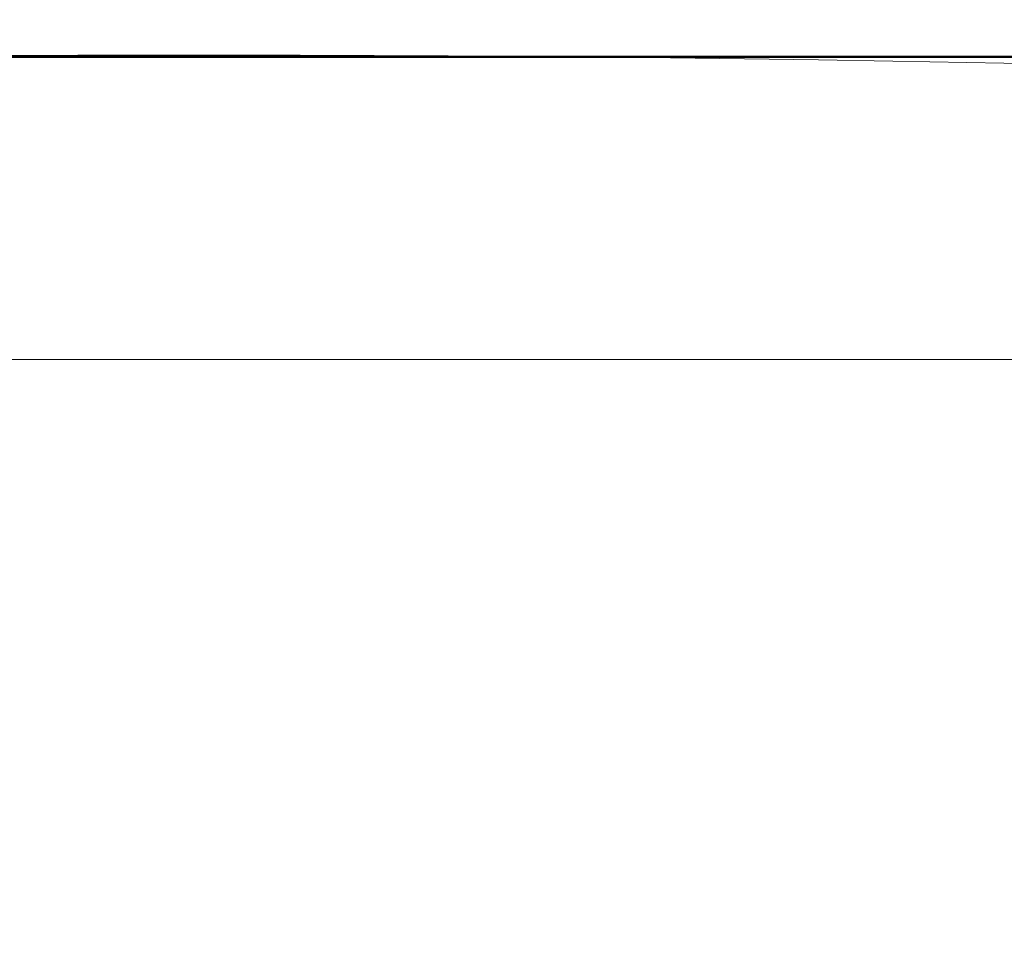
# Model space of a CAD drawing. Units: inches. Extents: x -466983 to 1020, y 324 to 318697.
# Tile 73 of 97: x 643.839 to 650.415, y 947.975 to 954.185. Entities that reach past the tile are written whole.
import ezdxf

# ---------------------------------------------------------------- set-up
doc = ezdxf.new("R2010")
doc.units = ezdxf.units.IN
doc.header["$MEASUREMENT"] = 0
for name, color, linetype, lineweight in [('A-FLOR-PATT', 252, 'Continuous', 13), ('A-FURN', 8, 'Continuous', 18), ('A-WALL', 7, 'Continuous', 50)]:
    doc.layers.add(name, color=color, linetype=linetype, lineweight=lineweight)

# ---------------------------------------------------------------- blocks, each defined once
blk = doc.blocks.new('L Shaped Sofa')
at = {"ltscale": 2}
for p, q in [((2430.914, 726.917), (2396.145, 726.917)), ((2475.263, 723.229), (2377.232, 723.229))]:
    blk.add_line(p, q, dxfattribs=at)
blk.add_arc((2416.36, 1205.029), 481.82, 262.88673, 276.63201, dxfattribs=at)

msp = doc.modelspace()

# ---------------------------------------------------------------- hatches: boundary and pattern name
at = {"layer": 'A-FLOR-PATT', "transparency": 33554572}
h = msp.add_hatch(dxfattribs=at)
h.set_pattern_fill('ANSI37', color=256, scale=30)
h.set_pattern_definition([(45, (-1212.4137, -290.035), (-2.6516504, 2.6516504), []), (135, (-1212.4137, -290.035), (-2.6516504, -2.6516504), [])])
h.paths.add_polyline_path([(901.8057, 1075.9377), (900.6144, 1075.9377), (900.6144, 1065.3856), (899.391, 1065.3856), (898.0911, 1065.3856), (892.8356, 1058.7098, -0.258377), (892.1875, 1058.3509), (879.9848, 1058.3509, -0.20177), (879.4382, 1058.5808), (874.0812, 1065.3856), (872.7813, 1065.3856), (871.5579, 1065.3856), (871.5579, 1075.9377), (813.8057, 1075.9377), (813.8057, 1044.7922), (832.3947, 1044.7922, -0.394795), (848.6602, 1028.5356), (848.6602, 1009.9377), (901.8057, 1009.9377), (901.8057, 1015.9377), (901.3057, 1015.9377), (871.3057, 1015.9377), (871.3057, 1017.2502), (871.3344, 1017.2502, -0.401453), (901.3057, 1045.9377), (901.8057, 1045.9377)])
edge = h.paths.add_edge_path(flags=16)
edge.add_line((847.7731, 1068.9486), (847.7731, 1073.7088))
edge.add_arc((849.2269, 1073.7088), 1.4538, 90, 180, ccw=False)
edge.add_line((849.2269, 1075.1627), (864.4921, 1075.1627))
edge.add_arc((864.4921, 1073.7088), 1.4538, 0, 90, ccw=False)
edge.add_line((865.9459, 1073.7088), (865.9459, 1069.0035))
edge.add_arc((832.6447, 1068.9761), 33.3012, -20.61234, 0.04725, ccw=False)
edge.add_ellipse((856.8595, 1058.48), major_axis=(0, 10.2131), ratio=0.6859192, start_angle=100.00884, end_angle=259.99116, ccw=False)
edge.add_arc((881.0742, 1068.9761), 33.3012, 180.04725, 200.61234, ccw=False)
h.paths.add_polyline_path([(853.1456, 1066.4815), (853.1456, 1066.4534), (853.1463, 1066.4534, 0.433107), (852.9166, 1066.6849), (852.9166, 1066.4534), (853.1456, 1066.4534), (853.1456, 1066.4815), (853.088, 1066.6122, 0.697939), (852.6995, 1066.4534), (852.7003, 1066.4534), (852.7003, 1066.4815), (852.9166, 1067.0012), (852.9166, 1066.6849, -0.396254)], flags=0)
h.paths.add_polyline_path([(861.0187, 1066.4815), (861.0187, 1066.4534), (861.0194, 1066.4534, 0.416404), (860.8024, 1066.6849), (860.8024, 1066.4534), (861.0187, 1066.4534), (861.0187, 1066.4815), (860.9672, 1066.6053, 0.713344), (860.5726, 1066.4534), (860.5734, 1066.4534), (860.5734, 1066.4815), (860.8024, 1067.0012), (860.8024, 1066.6849, -0.379973)], flags=0)
edge = h.paths.add_edge_path(flags=0)
edge.add_spline(control_points=[(861.1298, 1065.7855), (861.4661, 1065.2478), (861.6134, 1065.0161), (861.9833, 1064.3736), (862.1924, 1063.9443), (862.5614, 1063.0391), (862.7212, 1062.5633), (862.9865, 1061.5781), (863.092, 1061.0689), (863.2452, 1060.031), (863.293, 1059.5025), (863.3295, 1058.4409), (863.3181, 1057.9078), (863.2366, 1056.8518), (863.1664, 1056.3289), (862.9695, 1055.308), (862.8427, 1054.8099), (862.5365, 1053.8522), (862.3571, 1053.3927), (861.9514, 1052.5249), (861.7251, 1052.1166), (861.233, 1051.3622), (860.9672, 1051.0162), (860.4048, 1050.3949), (860.1082, 1050.1197), (859.4937, 1049.6461), (859.1758, 1049.4476), (858.5276, 1049.1299), (858.1973, 1049.0107), (857.5315, 1048.8518), (857.1959, 1048.8121), (856.5249, 1048.812), (856.1894, 1048.8515), (855.5236, 1049.0101), (855.1933, 1049.1291), (854.545, 1049.4465), (854.2271, 1049.6449), (853.6124, 1050.1183), (853.3158, 1050.3933), (852.7533, 1051.0143), (852.4874, 1051.3602), (851.9952, 1052.1144), (851.7688, 1052.5225), (851.3629, 1053.3902), (851.1834, 1053.8496), (850.877, 1054.8071), (850.7501, 1055.3051), (850.553, 1056.326), (850.4827, 1056.8488), (850.401, 1057.9048), (850.3895, 1058.4379), (850.4257, 1059.4995), (850.4734, 1060.0281), (850.6265, 1061.066), (850.7318, 1061.5753), (850.9969, 1062.5605), (851.1567, 1063.0365), (851.5254, 1063.9418), (851.7345, 1064.3712), (852.1056, 1065.0164), (852.2544, 1065.2503), (852.6082, 1065.7335)], knot_values=[3.915332, 3.915332, 3.915332, 3.915332, 4.013468, 4.013468, 4.175532, 4.175532, 4.337596, 4.337596, 4.49966, 4.49966, 4.661724, 4.661724, 4.823788, 4.823788, 4.985852, 4.985852, 5.147916, 5.147916, 5.30998, 5.30998, 5.472044, 5.472044, 5.634109, 5.634109, 5.796173, 5.796173, 5.958237, 5.958237, 6.120301, 6.120301, 6.282365, 6.282365, 6.444429, 6.444429, 6.606493, 6.606493, 6.768557, 6.768557, 6.930621, 6.930621, 7.092685, 7.092685, 7.254749, 7.254749, 7.416813, 7.416813, 7.578878, 7.578878, 7.740942, 7.740942, 7.903006, 7.903006, 8.06507, 8.06507, 8.227134, 8.227134, 8.389198, 8.389198, 8.551262, 8.551262, 8.65037, 8.65037, 8.65037, 8.65037], degree=3, periodic=0)
edge.add_line((852.6421, 1065.7855), (861.1298, 1065.7855))
edge = h.paths.add_edge_path(flags=0)
edge.add_ellipse((856.8496, 1057.7432), major_axis=(0, 7.7921), ratio=0.687861, start_angle=0, end_angle=360)
h.paths.add_polyline_path([(848.8634, 1069.3891), (848.8634, 1073.9605, -0.414214), (849.9538, 1075.0508), (863.7652, 1075.0508, -0.414214), (864.8555, 1073.9605), (864.8555, 1069.3891, -0.388936), (864.5237, 1069.027, -0.043561), (849.1953, 1069.027, -0.388936)], flags=0)
h.paths.add_polyline_path([(853.1006, 1068.1122, -1), (852.6775, 1068.1122, -1)], flags=0)
edge = h.paths.add_edge_path(flags=0)
edge.add_ellipse((856.8595, 1057.3378), major_axis=(0, 2.207), ratio=0.657164, start_angle=0, end_angle=360)
h.paths.add_polyline_path([(861.0415, 1068.1122, -1), (860.6184, 1068.1122, -1)], flags=0)
edge = h.paths.add_edge_path()
edge.add_line((573.9537, 1057.3412), (573.9537, 1075.9377))
edge.add_line((573.9537, 1075.9377), (558.7308, 1075.9377))
edge.add_line((558.7308, 1075.9377), (558.7308, 1065.3856))
edge.add_line((558.7308, 1065.3856), (557.5074, 1065.3856))
edge.add_line((557.5074, 1065.3856), (556.2075, 1065.3856))
edge.add_line((556.2075, 1065.3856), (550.952, 1058.7098))
edge.add_arc((550.3039, 1059.1155), 0.7646, 270, 327.94832, ccw=False)
edge.add_line((550.3039, 1058.3509), (538.1012, 1058.3509))
edge.add_arc((538.1012, 1059.1155), 0.7646, 224.3704, 270, ccw=False)
edge.add_line((537.5546, 1058.5808), (532.1976, 1065.3856))
edge.add_line((532.1976, 1065.3856), (530.8977, 1065.3856))
edge.add_line((530.8977, 1065.3856), (529.6743, 1065.3856))
edge.add_line((529.6743, 1065.3856), (529.6743, 1075.9377))
edge.add_line((529.6743, 1075.9377), (520.8057, 1075.9377))
edge.add_line((520.8057, 1075.9377), (520.8057, 1045.9377))
edge.add_line((520.8057, 1045.9377), (521.3057, 1045.9377))
edge.add_arc((521.3057, 1015.9377), 30, 2.50749, 90, ccw=False)
edge.add_line((551.277, 1017.2502), (551.3057, 1017.2502))
edge.add_line((551.3057, 1017.2502), (551.3057, 1015.9377))
edge.add_line((551.3057, 1015.9377), (520.8057, 1015.9377))
edge.add_line((520.8057, 1015.9377), (520.8057, 1009.9377))
edge.add_line((520.8057, 1009.9377), (559.1913, 1010.4022))
edge.add_arc((559.1913, 1011.856), 1.4538, 180, 270, ccw=False)
edge.add_line((557.7375, 1011.856), (557.7375, 1016.5613))
edge.add_arc((591.0386, 1016.5888), 33.3012, 159.38766, 180.04725, ccw=False)
edge.add_ellipse((566.8239, 1027.0848), major_axis=(0, 10.2131), ratio=0.6859192, start_angle=280.00884, end_angle=439.99116, ccw=False)
edge.add_arc((542.6091, 1016.5888), 33.3012, 0.04725, 20.61234, ccw=False)
edge.add_line((575.9103, 1016.6162), (575.9103, 1011.856))
edge.add_arc((574.4565, 1011.856), 1.4538, -90, 0, ccw=False)
edge.add_line((574.4565, 1010.4022), (608.8057, 1009.9377))
edge.add_line((608.8057, 1009.9377), (608.8057, 1041.0857))
edge.add_line((608.8057, 1041.0857), (590.2179, 1041.0857))
edge.add_arc((590.775, 1057.9074), 16.8309, 181.92775, 268.10321, ccw=False)
edge = h.paths.add_edge_path()
edge.add_ellipse((494.2443, 583.6204), major_axis=(0, 10.2131), ratio=0.6859192, start_angle=280.00884, end_angle=439.99116, ccw=False)
edge.add_arc((470.0296, 573.1243), 33.3012, 0.04725, 20.61234, ccw=False)
edge.add_line((503.3307, 573.1518), (503.3307, 568.3916))
edge.add_arc((501.8769, 568.3916), 1.4538, -90, 0, ccw=False)
edge.add_line((501.8769, 566.9377), (539.8057, 566.9377))
edge.add_line((539.8057, 566.9377), (539.8057, 572.9377))
edge.add_line((539.8057, 572.9377), (539.3057, 572.9377))
edge.add_line((539.3057, 572.9377), (509.3057, 572.9377))
edge.add_line((509.3057, 572.9377), (509.3057, 574.2502))
edge.add_line((509.3057, 574.2502), (509.3344, 574.2502))
edge.add_arc((539.3057, 572.9377), 30, 90, 177.49251, ccw=False)
edge.add_line((539.3057, 602.9377), (539.8057, 602.9377))
edge.add_line((539.8057, 602.9377), (539.8057, 626.9377))
edge.add_line((539.8057, 626.9377), (531.7718, 626.9377))
edge.add_line((531.7718, 626.9377), (531.7718, 616.3856))
edge.add_line((531.7718, 616.3856), (530.5484, 616.3856))
edge.add_line((530.5484, 616.3856), (529.2485, 616.3856))
edge.add_line((529.2485, 616.3856), (523.7105, 609.3509))
edge.add_line((523.7105, 609.3509), (510.7766, 609.3509))
edge.add_line((510.7766, 609.3509), (505.2386, 616.3856))
edge.add_line((505.2386, 616.3856), (503.9387, 616.3856))
edge.add_line((503.9387, 616.3856), (502.7153, 616.3856))
edge.add_line((502.7153, 616.3856), (502.7153, 626.9377))
edge.add_line((502.7153, 626.9377), (481.6983, 626.9377))
edge.add_line((481.6983, 626.9377), (481.6983, 610.995))
edge.add_arc((467.2703, 611.4728), 14.4359, 271.92775, 358.10321, ccw=False)
edge.add_line((467.7559, 597.0451), (451.8057, 597.0451))
edge.add_line((451.8057, 597.0451), (451.8057, 584.4035))
edge.add_line((451.8057, 584.4035), (451.8057, 566.9377))
edge.add_line((451.8057, 566.9377), (486.6117, 566.9377))
edge.add_arc((486.6117, 568.3916), 1.4538, 180, 270, ccw=False)
edge.add_line((485.1579, 568.3916), (485.1579, 573.0969))
edge.add_arc((518.4591, 573.1243), 33.3012, 159.38766, 180.04725, ccw=False)
h.paths.add_polyline_path([(836.2609, 1020.7328), (879.8898, 1020.7328), (879.8898, 1039.3902), (836.2609, 1039.3902)], flags=25)
h.paths.add_polyline_path([(549.9851, 1036.7492), (593.614, 1036.7492), (593.614, 1055.4065), (549.9851, 1055.4065)], flags=24)
h.paths.add_polyline_path([(475.123, 595.5959), (518.752, 595.5959), (518.752, 614.2532), (475.123, 614.2532)], flags=24)
h = msp.add_hatch(dxfattribs=at)
h.set_pattern_fill('ANSI37', color=256, scale=20)
h.set_pattern_definition([(45, (-1212.4137, -290.035), (-1.767767, 1.767767), []), (135, (-1212.4137, -290.035), (-1.767767, -1.767767), [])])
h.paths.add_polyline_path([(809.8057, 870.9377), (809.8057, 888.1519), (806.9985, 888.1519), (802.6624, 888.1519), (789.3832, 888.1519), (786.2846, 888.1519, -0.414214), (785.4991, 888.9374), (785.4991, 900.1959), (785.4991, 908.4696, -0.414214), (786.8082, 909.7787, -0.414214), (785.4991, 911.0878), (785.4991, 929.1015, -0.414214), (786.8082, 930.4106, -0.414214), (785.4991, 931.7197), (785.4991, 931.9039, -0.414214), (784.19, 930.5948), (766.7223, 930.5948, -0.412359), (765.4132, 931.8956, -0.413741), (764.1145, 930.5782), (744.5781, 930.422, -0.416556), (743.7864, 931.2075), (743.7864, 933.5153), (742.2154, 933.5153), (742.2154, 952.024, -0.001344), (743.7864, 952.1998), (743.7864, 953.9377), (678.5915, 953.9377), (678.5915, 951.1305), (678.5915, 946.7945), (678.5915, 933.5153), (678.5915, 930.4166, -0.414214), (677.806, 929.6312), (666.5475, 929.6312), (658.2738, 929.6312, -0.414214), (656.9647, 930.9403, -0.414214), (655.6556, 929.6312), (637.6419, 929.6312, -0.414214), (636.3328, 930.9403, -0.414214), (635.0237, 929.6312), (634.8395, 929.6312, -0.414214), (636.1486, 928.322), (636.1486, 910.8544, -0.412359), (634.8478, 909.5452, -0.413741), (636.1653, 908.2466), (636.3214, 888.7102, -0.416556), (635.5359, 887.9184), (633.2281, 887.9184), (633.2281, 886.3475), (614.7194, 886.3475, -0.001344), (614.5436, 887.9184), (612.8057, 887.9184), (612.8057, 834.9377), (612.8057, 752.9377), (612.8057, 748.9377), (612.8057, 697.9377), (654.8057, 697.9377), (654.8057, 701.9377), (715.8057, 701.9377), (715.8057, 737.4353), (774.2918, 737.4353), (774.2918, 795.9377), (809.8057, 795.9377)])
h.paths.add_polyline_path([(679.2761, 849.5757, 0.102523), (682.1475, 849.2608, -0.080461), (694.5428, 849.7725, -0.283899), (694.4822, 849.0082, 0.136605), (694.4068, 848.8103, -0.030441), (694.5428, 846.8929), (694.5428, 842.6198), (694.5428, 838.3466, -0.028219), (694.4246, 836.5684), (694.425, 836.5684, 0.196187), (694.4456, 836.2708, -0.302897), (694.5428, 835.467, -0.080461), (682.1475, 835.9787, 0.102523), (679.2761, 835.6638, -0.58611), (678.6457, 836.0169), (678.6457, 849.2227, -0.58611)], flags=16)
h.paths.add_polyline_path([(679.5173, 848.6515, 0.699597), (679.476, 848.6342, 1.20716), (679.1935, 848.7422, 0.010621)], flags=0)
h.paths.add_polyline_path([(679.4923, 836.5608, -0.013798), (679.9178, 836.6594, -0.071703), (682.8533, 837.1434, -0.165743), (682.1665, 839.1006), (682.1665, 842.6094), (682.1665, 846.0603, -0.240616), (683.4733, 848.6767, -0.068263), (693.9295, 849.0082), (693.7875, 848.7083), (693.7875, 849.0228, 0.067332), (683.4733, 848.6767, 0.240616), (682.1665, 846.0603), (682.1665, 842.6094), (682.1665, 839.1006, 0.23459), (683.461, 836.5513, 0.068093), (693.7875, 836.1955), (693.7875, 836.5104), (693.9296, 836.2102, -0.077215), (682.2421, 836.7815, 0.086627), (679.5283, 836.5701, -0.628402), (679.5029, 836.5735), (679.5029, 836.6071, 0.910458)], flags=0)
h.paths.add_polyline_path([(679.476, 848.6364), (679.2069, 848.647), (679.2069, 836.5718, 0.913566), (679.3645, 836.5861), (679.476, 836.5824)], flags=0)
h.paths.add_polyline_path([(679.2761, 829.8604, 0.102523), (682.1475, 829.5455, -0.080461), (694.5428, 830.0572, -0.283899), (694.4822, 829.2929, 0.136605), (694.4068, 829.095, -0.030441), (694.5428, 827.1776), (694.5428, 822.9045), (694.5428, 818.6314, -0.028219), (694.4246, 816.8531), (694.425, 816.8532, 0.196187), (694.4456, 816.5555, -0.302897), (694.5428, 815.7517, -0.080461), (682.1475, 816.2635, 0.102523), (679.2761, 815.9485, -0.58611), (678.6457, 816.3016), (678.6457, 829.5074, -0.58611)], flags=16)
h.paths.add_polyline_path([(679.5173, 828.9362, 0.699597), (679.476, 828.9189, 1.20716), (679.1935, 829.0269, 0.010621)], flags=0)
h.paths.add_polyline_path([(679.4923, 816.8456, -0.013798), (679.9178, 816.9441, -0.071703), (682.8533, 817.4281, -0.165743), (682.1665, 819.3853), (682.1665, 822.8941), (682.1665, 826.345, -0.240616), (683.4733, 828.9614, -0.068263), (693.9295, 829.2929), (693.7875, 828.9931), (693.7875, 829.3076, 0.067332), (683.4733, 828.9614, 0.240616), (682.1665, 826.345), (682.1665, 822.8941), (682.1665, 819.3853, 0.23459), (683.461, 816.836, 0.068093), (693.7875, 816.4802), (693.7875, 816.7952), (693.9296, 816.4949, -0.077215), (682.2421, 817.0662, 0.086627), (679.5283, 816.8549, -0.628402), (679.5029, 816.8582), (679.5029, 816.8918, 0.910458)], flags=0)
h.paths.add_polyline_path([(679.476, 828.9211), (679.2069, 828.9317), (679.2069, 816.8565, 0.913566), (679.3645, 816.8708), (679.476, 816.8671)], flags=0)
h.paths.add_polyline_path([(679.2761, 810.1451, 0.102523), (682.1475, 809.8302, -0.080461), (694.5428, 810.342, -0.3023), (694.4466, 809.5394, 0.10023), (694.4058, 809.3878, -0.03057), (694.5428, 807.4623), (694.5428, 803.1892), (694.5428, 798.9161, -0.03057), (694.4058, 796.9906, 0.10023), (694.4466, 796.839, -0.3023), (694.5428, 796.0365, -0.080461), (682.1475, 796.5482, 0.102523), (679.2761, 796.2333, -0.58611), (678.6457, 796.5863), (678.6457, 809.7921, -0.58611)], flags=16)
h.paths.add_polyline_path([(679.5173, 809.2417, 0.699597), (679.476, 809.2244, 1.20716), (679.1935, 809.3324, 0.010621)], flags=0)
h.paths.add_polyline_path([(679.4923, 797.151, -0.013798), (679.9178, 797.2496, -0.071703), (682.8533, 797.7336, -0.165743), (682.1665, 799.6908), (682.1665, 803.1996), (682.1665, 806.6505, -0.239349), (683.461, 809.2577, -0.072465), (694.4468, 809.5405, 0.197932), (694.425, 809.2405), (693.7875, 809.2985), (693.7875, 809.6135, 0.068093), (683.461, 809.2577, 0.239349), (682.1665, 806.6505), (682.1665, 803.1996), (682.1665, 799.6908, 0.235854), (683.4733, 797.1323, 0.067332), (693.7875, 796.7861), (693.7875, 797.1006), (694.425, 797.1586, 0.197932), (694.4468, 796.8586, -0.080419), (682.1557, 797.3795, 0.083867), (679.5283, 797.1603, -0.628402), (679.5029, 797.1637), (679.5029, 797.1973, 0.910458)], flags=0)
h.paths.add_polyline_path([(679.2069, 809.2372), (679.2069, 797.162, 0.913566), (679.3645, 797.1763), (679.476, 797.1726), (679.476, 809.2266)], flags=0)
h.paths.add_polyline_path([(695.3643, 853.2989), (728.2231, 853.2989), (728.2231, 771.1519), (695.3643, 771.1519)], flags=16)
h.paths.add_polyline_path([(696.0215, 852.6417), (727.5659, 852.6417), (727.5659, 771.809), (696.0215, 771.809)], flags=0)
h.paths.add_polyline_path([(679.2761, 788.7869, 0.102523), (682.1475, 788.472, -0.080461), (694.5428, 788.9837, -0.3023), (694.4466, 788.1812, 0.10023), (694.4058, 788.0296, -0.03057), (694.5428, 786.1041), (694.5428, 781.831), (694.5428, 777.5578, -0.03057), (694.4058, 775.6323, 0.10023), (694.4466, 775.4808, -0.3023), (694.5428, 774.6782, -0.080461), (682.1475, 775.19, 0.102523), (679.2761, 774.875, -0.58611), (678.6457, 775.2281), (678.6457, 788.4339, -0.58611)], flags=16)
h.paths.add_polyline_path([(679.5173, 787.8834, 0.699597), (679.476, 787.8662, 1.20716), (679.1935, 787.9742, 0.010621)], flags=0)
h.paths.add_polyline_path([(679.4923, 775.7928, -0.013798), (679.9178, 775.8914, -0.071703), (682.8533, 776.3753, -0.165743), (682.1665, 778.3325), (682.1665, 781.8414), (682.1665, 785.2922, -0.239349), (683.461, 787.8995, -0.072465), (694.4468, 788.1823, 0.197932), (694.425, 787.8823), (693.7875, 787.9403), (693.7875, 788.2553, 0.068093), (683.461, 787.8995, 0.239349), (682.1665, 785.2922), (682.1665, 781.8414), (682.1665, 778.3325, 0.235854), (683.4733, 775.7741, 0.067332), (693.7875, 775.4279), (693.7875, 775.7424), (694.425, 775.8004, 0.197932), (694.4468, 775.5004, -0.080419), (682.1557, 776.0212, 0.083867), (679.5283, 775.8021, -0.628402), (679.5029, 775.8054), (679.5029, 775.8391, 0.910458)], flags=0)
h.paths.add_polyline_path([(679.2069, 787.8789), (679.2069, 775.8038, 0.913566), (679.3645, 775.818), (679.476, 775.8144), (679.476, 787.8684)], flags=0)
h.paths.add_polyline_path([(704.641, 854.1204, -0.080461), (705.1527, 866.5157, 0.102523), (704.8378, 869.3871, -0.58611), (705.1908, 870.0174), (718.3966, 870.0174, -0.58611), (718.7496, 869.3871, 0.102523), (718.4347, 866.5157, -0.080461), (718.9465, 854.1204, -0.3023), (718.1439, 854.2166, 0.10023), (717.9924, 854.2574, -0.03057), (716.0668, 854.1204), (711.7937, 854.1204), (707.5206, 854.1204, -0.03057), (705.5951, 854.2574, 0.10023), (705.4435, 854.2166, -0.3023)], flags=16)
h.paths.add_polyline_path([(717.8462, 869.1459, 0.699597), (717.8289, 869.1872, 1.20716), (717.9369, 869.4697, 0.010621)], flags=0)
h.paths.add_polyline_path([(705.4631, 854.2164, -0.080419), (705.984, 866.5074, 0.083867), (705.7648, 869.1349, -0.628402), (705.7682, 869.1603), (705.8018, 869.1603, 0.910458), (705.7555, 869.1709, -0.013798), (705.8541, 868.7454, -0.071703), (706.3381, 865.8099, -0.165743), (708.2953, 866.4967), (711.8041, 866.4967), (715.255, 866.4967, -0.239349), (717.8622, 865.2022, -0.072465), (718.145, 854.2164, 0.197932), (717.845, 854.2382), (717.903, 854.8757), (718.218, 854.8757, 0.068093), (717.8622, 865.2022, 0.239349), (715.255, 866.4967), (711.8041, 866.4967), (708.2953, 866.4967, 0.235854), (705.7368, 865.1898, 0.067332), (705.3906, 854.8757), (705.7051, 854.8757), (705.7631, 854.2382, 0.197932)], flags=16)
h.paths.add_polyline_path([(705.7665, 869.4563, 0.913566), (705.7808, 869.2987), (705.7771, 869.1872), (717.8311, 869.1872), (717.8417, 869.4563)], flags=0)
h.paths.add_polyline_path([(729.0446, 842.6198), (729.0446, 846.8929, -0.03057), (729.1817, 848.8184, 0.10023), (729.1408, 848.9699, -0.3023), (729.0446, 849.7725, -0.080461), (741.4399, 849.2608, 0.102523), (744.3113, 849.5757, -0.58611), (744.9417, 849.2227), (744.9417, 836.0169, -0.58611), (744.3113, 835.6638, 0.102523), (741.4399, 835.9787, -0.080461), (729.0446, 835.467, -0.3023), (729.1408, 836.2696, 0.10023), (729.1817, 836.4211, -0.03057), (729.0446, 838.3466)], flags=16)
h.paths.add_polyline_path([(744.1115, 836.5846, 1.20716), (744.3939, 836.4766, 0.010621), (744.0701, 836.5673, 0.699597)], flags=0)
h.paths.add_polyline_path([(729.1407, 836.2684, 0.197932), (729.1624, 836.5684), (729.7999, 836.5104), (729.7999, 836.1955, 0.068093), (740.1264, 836.5513, 0.239349), (741.4209, 839.1585), (741.4209, 842.6094), (741.4209, 846.1182, 0.235854), (740.1141, 848.6767, 0.067332), (729.7999, 849.0228), (729.7999, 848.7083), (729.1624, 848.6503, 0.197932), (729.1407, 848.9504, -0.080419), (741.4317, 848.4295, 0.083867), (744.0591, 848.6486, -0.628402), (744.0845, 848.6453), (744.0845, 848.6117, 0.910458), (744.0951, 848.6579, -0.013798), (743.6696, 848.5594, -0.071703), (740.7341, 848.0754, -0.165743), (741.4209, 846.1182), (741.4209, 842.6094), (741.4209, 839.1585, -0.239349), (740.1264, 836.5513, -0.072465)], flags=0)
h.paths.add_polyline_path([(729.0446, 830.0572, -0.080461), (741.4399, 829.5455, 0.102523), (744.3113, 829.8604, -0.58611), (744.9417, 829.5074), (744.9417, 816.3016, -0.58611), (744.3113, 815.9485, 0.102523), (741.4399, 816.2635, -0.080461), (729.0446, 815.7517, -0.3023), (729.1408, 816.5543, 0.10023), (729.1817, 816.7058, -0.03057), (729.0446, 818.6314), (729.0446, 822.9045), (729.0446, 827.1776, -0.03057), (729.1817, 829.1031, 0.10023), (729.1408, 829.2547, -0.3023)], flags=16)
h.paths.add_polyline_path([(744.1115, 816.8693, 1.20716), (744.3939, 816.7613, 0.010621), (744.0701, 816.852, 0.699597)], flags=0)
h.paths.add_polyline_path([(729.1407, 829.2351, -0.080419), (741.4317, 828.7142, 0.083867), (744.0591, 828.9334, -0.628402), (744.0845, 828.93), (744.0845, 828.8964, 0.910458), (744.0951, 828.9427, -0.013798), (743.6696, 828.8441, -0.071703), (740.7341, 828.3601, -0.165743), (741.4209, 826.4029), (741.4209, 822.8941), (741.4209, 819.4432, -0.239349), (740.1264, 816.836, -0.072465), (729.1407, 816.5531, 0.197932), (729.1624, 816.8532), (729.7999, 816.7952), (729.7999, 816.4802, 0.068093), (740.1264, 816.836, 0.239349), (741.4209, 819.4432), (741.4209, 822.8941), (741.4209, 826.4029, 0.235854), (740.1141, 828.9614, 0.067332), (729.7999, 829.3076), (729.7999, 828.9931), (729.1624, 828.9351, 0.197932)], flags=16)
h.paths.add_polyline_path([(729.0446, 810.342, -0.080461), (741.4399, 809.8302, 0.102523), (744.3113, 810.1451, -0.58611), (744.9417, 809.7921), (744.9417, 796.5863, -0.58611), (744.3113, 796.2333, 0.102523), (741.4399, 796.5482, -0.080461), (729.0446, 796.0365, -0.283899), (729.1052, 796.8007, 0.136605), (729.1806, 796.9987, -0.030441), (729.0446, 798.9161), (729.0446, 803.1892), (729.0446, 807.4623, -0.028219), (729.1628, 809.2406), (729.1624, 809.2405, 0.196187), (729.1418, 809.5382, -0.302897)], flags=16)
h.paths.add_polyline_path([(744.1115, 797.1748, 1.20716), (744.3939, 797.0668, 0.010621), (744.0701, 797.1575, 0.699597)], flags=0)
h.paths.add_polyline_path([(741.3453, 809.0275, 0.086627), (744.0591, 809.2388, -0.628402), (744.0845, 809.2355), (744.0845, 809.2019, 0.910458), (744.0951, 809.2481, -0.013798), (743.6696, 809.1496, -0.071703), (740.7341, 808.6656, -0.165743), (741.4209, 806.7084), (741.4209, 803.1996), (741.4209, 799.7487, -0.240616), (740.1141, 797.1323, -0.068263), (729.658, 796.8008), (729.7999, 797.1006), (729.7999, 796.7861, 0.067332), (740.1141, 797.1323, 0.240616), (741.4209, 799.7487), (741.4209, 803.1996), (741.4209, 806.7084, 0.23459), (740.1264, 809.2577, 0.068093), (729.7999, 809.6135), (729.7999, 809.2985), (729.6578, 809.5988, -0.077215)], flags=0)
h.paths.add_polyline_path([(704.641, 770.3304, -0.283899), (705.4053, 770.2697, 0.136605), (705.6032, 770.1944, -0.030441), (707.5206, 770.3304), (711.7937, 770.3304), (716.0668, 770.3304, -0.028219), (717.8451, 770.2122), (717.845, 770.2126, 0.196187), (718.1427, 770.2331, -0.302897), (718.9465, 770.3304, -0.080461), (718.4347, 757.9351, 0.102523), (718.7496, 755.0637, -0.58611), (718.3966, 754.4333), (705.1908, 754.4333, -0.58611), (704.8378, 755.0637, 0.102523), (705.1527, 757.9351, -0.080461)], flags=16)
h.paths.add_polyline_path([(705.762, 755.3048, 0.699597), (705.7793, 755.2635, 1.20716), (705.6713, 754.9811, 0.010621)], flags=0)
h.paths.add_polyline_path([(705.4053, 769.717), (705.7051, 769.5751), (705.3906, 769.5751, 0.067332), (705.7368, 759.2609, 0.240616), (708.3532, 757.954), (711.8041, 757.954), (715.3129, 757.954, 0.23459), (717.8622, 759.2485, 0.068093), (718.218, 769.5751), (717.903, 769.5751), (718.2033, 769.7172, -0.077215), (717.632, 758.0297, 0.086627), (717.8433, 755.3159, -0.628402), (717.84, 755.2904), (717.8064, 755.2904, 0.910458), (717.8526, 755.2799, -0.013798), (717.7541, 755.7053, -0.071703), (717.2701, 758.6409, -0.165743), (715.3129, 757.954), (711.8041, 757.954), (708.3532, 757.954, -0.240616), (705.7368, 759.2609, -0.068263)], flags=0)
h.paths.add_polyline_path([(729.0446, 788.9837, -0.080461), (741.4399, 788.472, 0.102523), (744.3113, 788.7869, -0.58611), (744.9417, 788.4339), (744.9417, 775.2281, -0.58611), (744.3113, 774.875, 0.102523), (741.4399, 775.19, -0.080461), (729.0446, 774.6782, -0.283899), (729.1052, 775.4425, 0.136605), (729.1806, 775.6405, -0.030441), (729.0446, 777.5578), (729.0446, 781.831), (729.0446, 786.1041, -0.028219), (729.1628, 787.8823), (729.1624, 787.8823, 0.196187), (729.1418, 788.1799, -0.302897)], flags=16)
h.paths.add_polyline_path([(744.1115, 775.8165, 1.20716), (744.3939, 775.7086, 0.010621), (744.0701, 775.7993, 0.699597)], flags=0)
h.paths.add_polyline_path([(741.3453, 787.6692, 0.086627), (744.0591, 787.8806, -0.628402), (744.0845, 787.8773), (744.0845, 787.8437, 0.910458), (744.0951, 787.8899, -0.013798), (743.6696, 787.7913, -0.071703), (740.7341, 787.3074, -0.165743), (741.4209, 785.3502), (741.4209, 781.8414), (741.4209, 778.3905, -0.240616), (740.1141, 775.7741, -0.068263), (729.658, 775.4425), (729.7999, 775.7424), (729.7999, 775.4279, 0.067332), (740.1141, 775.7741, 0.240616), (741.4209, 778.3905), (741.4209, 781.8414), (741.4209, 785.3502, 0.23459), (740.1264, 787.8995, 0.068093), (729.7999, 788.2553), (729.7999, 787.9403), (729.6578, 788.2405, -0.077215)], flags=0)
h.paths.add_polyline_path([(744.1115, 848.6364), (744.1115, 836.5824), (744.3805, 836.5718), (744.3805, 848.647, 0.913566), (744.2229, 848.6327)], flags=0)
h.paths.add_polyline_path([(744.2229, 828.9174), (744.1115, 828.9211), (744.1115, 816.8671), (744.3805, 816.8565), (744.3805, 828.9317, 0.913566)], flags=0)
h.paths.add_polyline_path([(717.8311, 755.2635), (705.7771, 755.2635), (705.7665, 754.9945), (717.8417, 754.9945, 0.913566), (717.8274, 755.1521)], flags=0)
h.paths.add_polyline_path([(744.2229, 809.2229), (744.1115, 809.2266), (744.1115, 797.1726), (744.3805, 797.162), (744.3805, 809.2372, 0.913566)], flags=0)
h.paths.add_polyline_path([(744.1115, 787.8684), (744.1115, 775.8144), (744.3805, 775.8038), (744.3805, 787.8789, 0.913566), (744.2229, 787.8647)], flags=0)
h.paths.add_polyline_path([(678.8774, 877.1228), (737.6127, 877.1228), (737.6127, 899.5116), (678.8774, 899.5116)], flags=24)

# ---------------------------------------------------------------- linework, layer by layer
at = {"layer": 'A-FURN', "ltscale": 2}
for p, q in [((612.8057, 953.9377), (666.5475, 953.9377)), ((612.8057, 953.9377), (666.5475, 953.9377)), ((612.8057, 953.9377), (666.5475, 953.9377)), ((612.8057, 953.9377), (666.5475, 953.9377)), ((612.8057, 953.9377), (666.5475, 953.9377)), ((612.8057, 953.9377), (666.5475, 953.9377)), ((637.1183, 951.916), (656.1792, 951.916)), ((637.1183, 951.916), (656.1792, 951.916)), ((637.1183, 951.916), (656.1792, 951.916)), ((637.1183, 951.916), (656.1792, 951.916)), ((637.1183, 951.916), (656.1792, 951.916)), ((637.1183, 951.916), (656.1792, 951.916))]:
    msp.add_line(p, q, dxfattribs=at)
msp.add_arc((645.0971, 689.8078), 264.1412, 82.88673, 96.632015, dxfattribs=at)
msp.add_arc((645.0971, 689.8078), 264.1412, 82.88673, 96.632015, dxfattribs=at)
msp.add_arc((645.0971, 689.8078), 264.1412, 82.88673, 96.632015, dxfattribs=at)
msp.add_arc((645.0971, 689.8078), 264.1412, 82.88673, 96.632015, dxfattribs=at)
msp.add_arc((645.0971, 689.8078), 264.1412, 82.88673, 96.632015, dxfattribs=at)
msp.add_arc((645.0971, 689.8078), 264.1412, 82.88673, 96.632015, dxfattribs=at)
at = {"layer": 'A-WALL'}
msp.add_line((612.8057, 953.9377), (680.5915, 953.9377), dxfattribs=at)

# ---------------------------------------------------------------- block references
at = {"layer": 'A-FURN', "xscale": 0.5482153745360612, "yscale": 0.5482153745360612, "zscale": 0.5482153745360612, "rotation": 180}
msp.add_blockref('L Shaped Sofa', (1969.7828, 1350.4232), dxfattribs=at)

doc.saveas('drawing.dxf')
